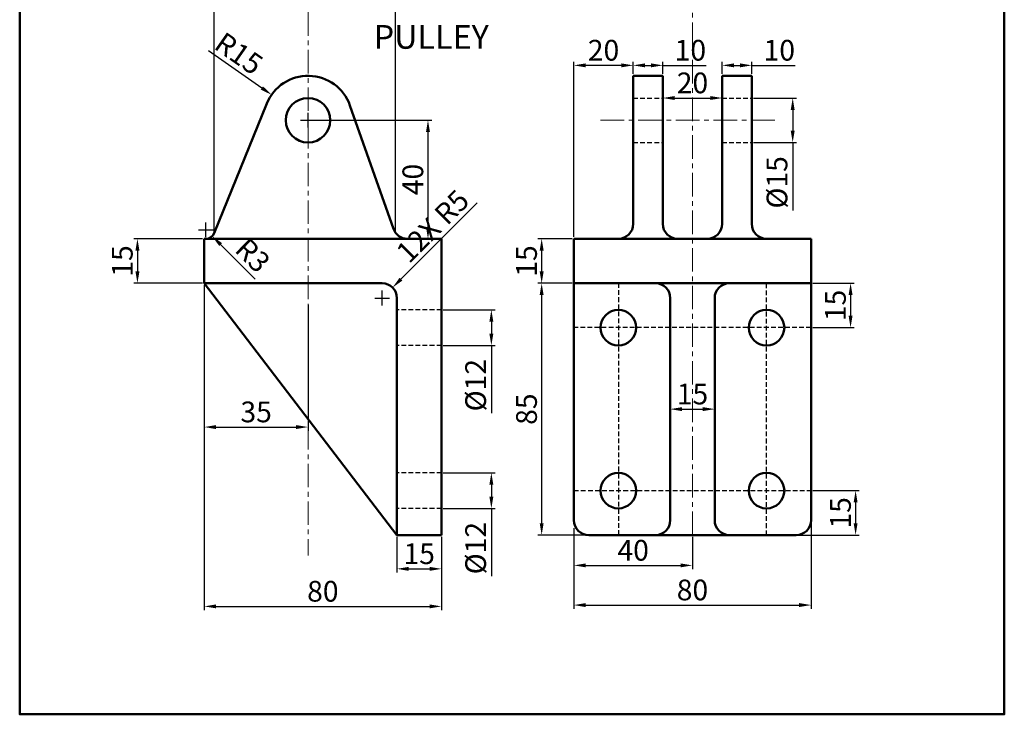
# Model space of a CAD drawing. Units: millimetres. Extents: x 50 to 393, y 3 to 474.
# Tile 1 of 2: x 61 to 393, y 3 to 238. Entities that reach past the tile are written whole.
import ezdxf

# ---------------------------------------------------------------- set-up
doc = ezdxf.new("R2010")
doc.units = ezdxf.units.MM
doc.header["$LTSCALE"] = 0.5
doc.linetypes.add('CENTER', pattern=[50.8, 31.75, -6.35, 6.35, -6.35])
doc.linetypes.add('HIDDEN', pattern=[9.525, 6.35, -3.175])
for name, color, linetype, lineweight in [('M-CNTR', 4, 'CENTER', 18), ('M-DIMS', 2, 'Continuous', 25), ('M-HIDN', 1, 'HIDDEN', 25), ('M-OUTL', 7, 'Continuous', 50), ('M-TEXT', 7, 'Continuous', 25), ('M-TTLB', 7, 'Continuous', 50)]:
    doc.layers.add(name, color=color, linetype=linetype, lineweight=lineweight)
doc.styles.get("Standard").update_dxf_attribs({"font": 'arial.ttf'})
doc.dimstyles.new('ISO-25', dxfattribs={"dimtxt": 7, "dimasz": 4, "dimexe": 1.25, "dimexo": 0.625, "dimtad": 1, "dimtxsty": 'Standard', "dimcen": 2.5, "dimadec": 0, "dimazin": 0, "dimtfac": 1, "dimtofl": 0, "dimtmove": 0, "dimatfit": 3, "dimfxl": 1, "dimarcsym": 0})

# ---------------------------------------------------------------- blocks, each defined once
blk = doc.blocks.new('*D1')
at = {"layer": 'Defpoints', "color": 0, "ltscale": 0.5, "transparency": 16777216}
for p in [(122.79, 163.96), (100.24, 148.96), (122.79, 148.96)]:
    blk.add_point(p, dxfattribs=at)
at = {"layer": 'M-DIMS', "color": 0, "lineweight": -2, "ltscale": 0.5, "transparency": 16777216}
for p, q in [((122.16, 163.96), (98.99, 163.96)), ((100.24, 159.96), (100.24, 152.96)), ((122.16, 148.96), (98.99, 148.96))]:
    blk.add_line(p, q, dxfattribs=at)
at = {"layer": 'M-DIMS', "color": 0, "ltscale": 0.5, "transparency": 16777216}
for points in [[(99.58, 159.96), (100.91, 159.96), (100.24, 163.96)], [(99.58, 152.96), (100.91, 152.96), (100.24, 148.96)]]:
    blk.add_solid(points, dxfattribs=at)
at = {"layer": 'M-DIMS', "color": 0, "ltscale": 0.5, "transparency": 16777216, "insert": (96.04, 156.46), "char_height": 7, "attachment_point": 5, "rotation": 90}
blk.add_mtext('15', dxfattribs=at)
blk = doc.blocks.new('*D2')
at = {"layer": 'Defpoints', "color": 0, "ltscale": 0.5, "transparency": 16777216}
for p in [(122.79, 148.96), (157.79, 142.23), (157.79, 100.41)]:
    blk.add_point(p, dxfattribs=at)
at = {"layer": 'M-DIMS', "color": 0, "lineweight": -2, "ltscale": 0.5, "transparency": 16777216}
for p, q in [((122.79, 148.34), (122.79, 99.16)), ((157.79, 141.61), (157.79, 99.16)), ((126.79, 100.41), (153.79, 100.41))]:
    blk.add_line(p, q, dxfattribs=at)
at = {"layer": 'M-DIMS', "color": 0, "ltscale": 0.5, "transparency": 16777216}
for points in [[(126.79, 101.07), (126.79, 99.74), (122.79, 100.41)], [(153.79, 101.07), (153.79, 99.74), (157.79, 100.41)]]:
    blk.add_solid(points, dxfattribs=at)
at = {"layer": 'M-DIMS', "color": 0, "ltscale": 0.5, "transparency": 16777216, "insert": (140.29, 104.61), "char_height": 7, "attachment_point": 5}
blk.add_mtext('35', dxfattribs=at)
blk = doc.blocks.new('*D3')
at = {"layer": 'Defpoints', "color": 0, "ltscale": 0.5, "transparency": 16777216}
for p in [(122.79, 148.96), (202.79, 63.96), (202.79, 39.89)]:
    blk.add_point(p, dxfattribs=at)
at = {"layer": 'M-DIMS', "color": 0, "lineweight": -2, "ltscale": 0.5, "transparency": 16777216}
for p, q in [((122.79, 148.34), (122.79, 38.64)), ((202.79, 63.34), (202.79, 38.64)), ((126.79, 39.89), (198.79, 39.89))]:
    blk.add_line(p, q, dxfattribs=at)
at = {"layer": 'M-DIMS', "color": 0, "ltscale": 0.5, "transparency": 16777216}
for points in [[(126.79, 40.55), (126.79, 39.22), (122.79, 39.89)], [(198.79, 40.55), (198.79, 39.22), (202.79, 39.89)]]:
    blk.add_solid(points, dxfattribs=at)
at = {"layer": 'M-DIMS', "color": 0, "ltscale": 0.5, "transparency": 16777216, "insert": (162.79, 44.09), "char_height": 7, "attachment_point": 5}
blk.add_mtext('80', dxfattribs=at)
blk = doc.blocks.new('*D4')
at = {"layer": 'Defpoints', "color": 0, "ltscale": 0.5, "transparency": 16777216}
for p in [(187.79, 63.96), (202.79, 63.96), (202.79, 52.56)]:
    blk.add_point(p, dxfattribs=at)
at = {"layer": 'M-DIMS', "color": 0, "lineweight": -2, "ltscale": 0.5, "transparency": 16777216}
for p, q in [((187.79, 63.34), (187.79, 51.31)), ((202.79, 63.34), (202.79, 51.31)), ((191.79, 52.56), (198.79, 52.56))]:
    blk.add_line(p, q, dxfattribs=at)
at = {"layer": 'M-DIMS', "color": 0, "ltscale": 0.5, "transparency": 16777216}
for points in [[(191.79, 53.23), (191.79, 51.89), (187.79, 52.56)], [(198.79, 53.23), (198.79, 51.89), (202.79, 52.56)]]:
    blk.add_solid(points, dxfattribs=at)
at = {"layer": 'M-DIMS', "color": 0, "ltscale": 0.5, "transparency": 16777216, "insert": (195.29, 56.76), "char_height": 7, "attachment_point": 5}
blk.add_mtext('15', dxfattribs=at)
blk = doc.blocks.new('*D5')
at = {"layer": 'Defpoints', "color": 0, "ltscale": 0.5, "transparency": 16777216}
for p in [(157.79, 203.96), (157.79, 163.96), (198.26, 163.96)]:
    blk.add_point(p, dxfattribs=at)
at = {"layer": 'M-DIMS', "color": 0, "lineweight": -2, "ltscale": 0.5, "transparency": 16777216}
for p, q in [((158.41, 203.96), (199.51, 203.96)), ((198.26, 199.96), (198.26, 167.96)), ((158.41, 163.96), (199.51, 163.96))]:
    blk.add_line(p, q, dxfattribs=at)
at = {"layer": 'M-DIMS', "color": 0, "ltscale": 0.5, "transparency": 16777216}
for points in [[(197.59, 199.96), (198.92, 199.96), (198.26, 203.96)], [(197.59, 167.96), (198.92, 167.96), (198.26, 163.96)]]:
    blk.add_solid(points, dxfattribs=at)
at = {"layer": 'M-DIMS', "color": 0, "ltscale": 0.5, "transparency": 16777216, "insert": (194.06, 183.96), "char_height": 7, "attachment_point": 5, "rotation": 90}
blk.add_mtext('40', dxfattribs=at)
blk = doc.blocks.new('*D6')
at = {"layer": 'Defpoints', "color": 0, "ltscale": 0.5, "transparency": 16777216}
for p in [(202.79, 139.96), (202.79, 127.96), (219.64, 127.96)]:
    blk.add_point(p, dxfattribs=at)
at = {"layer": 'M-DIMS', "color": 0, "lineweight": -2, "ltscale": 0.5, "transparency": 16777216}
for p, q in [((203.41, 139.96), (220.89, 139.96)), ((219.64, 135.96), (219.64, 131.96)), ((203.41, 127.96), (220.89, 127.96)), ((219.64, 127.96), (219.64, 105.14))]:
    blk.add_line(p, q, dxfattribs=at)
at = {"layer": 'M-DIMS', "color": 0, "ltscale": 0.5, "transparency": 16777216}
for points in [[(218.97, 135.96), (220.31, 135.96), (219.64, 139.96)], [(218.97, 131.96), (220.31, 131.96), (219.64, 127.96)]]:
    blk.add_solid(points, dxfattribs=at)
at = {"layer": 'M-DIMS', "color": 0, "ltscale": 0.5, "transparency": 16777216, "insert": (215.24, 114.55), "char_height": 7, "attachment_point": 5, "rotation": 90}
blk.add_mtext('%%C12', dxfattribs=at)
blk = doc.blocks.new('*D7')
at = {"layer": 'Defpoints', "color": 0, "ltscale": 0.5, "transparency": 16777216}
for p in [(202.79, 84.96), (202.79, 72.96), (219.64, 72.96)]:
    blk.add_point(p, dxfattribs=at)
at = {"layer": 'M-DIMS', "color": 0, "lineweight": -2, "ltscale": 0.5, "transparency": 16777216}
for p, q in [((203.41, 84.96), (220.89, 84.96)), ((219.64, 80.96), (219.64, 76.96)), ((203.41, 72.96), (220.89, 72.96)), ((219.64, 72.96), (219.64, 50.14))]:
    blk.add_line(p, q, dxfattribs=at)
at = {"layer": 'M-DIMS', "color": 0, "ltscale": 0.5, "transparency": 16777216}
for points in [[(218.97, 80.96), (220.31, 80.96), (219.64, 84.96)], [(218.97, 76.96), (220.31, 76.96), (219.64, 72.96)]]:
    blk.add_solid(points, dxfattribs=at)
at = {"layer": 'M-DIMS', "color": 0, "ltscale": 0.5, "transparency": 16777216, "insert": (215.24, 59.55), "char_height": 7, "attachment_point": 5, "rotation": 90}
blk.add_mtext('%%C12', dxfattribs=at)
blk = doc.blocks.new('*D8')
at = {"layer": 'Defpoints', "color": 0, "ltscale": 0.5, "transparency": 16777216}
for p in [(247.48, 163.96), (236.61, 148.96), (247.48, 148.96)]:
    blk.add_point(p, dxfattribs=at)
at = {"layer": 'M-DIMS', "color": 0, "lineweight": -2, "ltscale": 0.5, "transparency": 16777216}
for p, q in [((246.86, 163.96), (235.36, 163.96)), ((236.61, 159.96), (236.61, 152.96)), ((246.86, 148.96), (235.36, 148.96))]:
    blk.add_line(p, q, dxfattribs=at)
at = {"layer": 'M-DIMS', "color": 0, "ltscale": 0.5, "transparency": 16777216}
for points in [[(235.94, 159.96), (237.28, 159.96), (236.61, 163.96)], [(235.94, 152.96), (237.28, 152.96), (236.61, 148.96)]]:
    blk.add_solid(points, dxfattribs=at)
at = {"layer": 'M-DIMS', "color": 0, "ltscale": 0.5, "transparency": 16777216, "insert": (232.41, 156.46), "char_height": 7, "attachment_point": 5, "rotation": 90}
blk.add_mtext('15', dxfattribs=at)
blk = doc.blocks.new('*D9')
at = {"layer": 'Defpoints', "color": 0, "ltscale": 0.5, "transparency": 16777216}
for p in [(247.48, 148.96), (236.61, 63.96), (252.48, 63.96)]:
    blk.add_point(p, dxfattribs=at)
at = {"layer": 'M-DIMS', "color": 0, "lineweight": -2, "ltscale": 0.5, "transparency": 16777216}
for p, q in [((246.86, 148.96), (235.36, 148.96)), ((236.61, 144.96), (236.61, 67.96)), ((251.86, 63.96), (235.36, 63.96))]:
    blk.add_line(p, q, dxfattribs=at)
at = {"layer": 'M-DIMS', "color": 0, "ltscale": 0.5, "transparency": 16777216}
for points in [[(235.94, 144.96), (237.28, 144.96), (236.61, 148.96)], [(235.94, 67.96), (237.28, 67.96), (236.61, 63.96)]]:
    blk.add_solid(points, dxfattribs=at)
at = {"layer": 'M-DIMS', "color": 0, "ltscale": 0.5, "transparency": 16777216, "insert": (232.41, 106.46), "char_height": 7, "attachment_point": 5, "rotation": 90}
blk.add_mtext('85', dxfattribs=at)
blk = doc.blocks.new('*D10')
at = {"layer": 'Defpoints', "color": 0, "ltscale": 0.5, "transparency": 16777216}
for p in [(247.48, 63.96), (287.48, 63.96), (287.48, 53.73)]:
    blk.add_point(p, dxfattribs=at)
at = {"layer": 'M-DIMS', "color": 0, "lineweight": -2, "ltscale": 0.5, "transparency": 16777216}
for p, q in [((247.48, 63.34), (247.48, 52.48)), ((287.48, 63.34), (287.48, 52.48)), ((251.48, 53.73), (283.48, 53.73))]:
    blk.add_line(p, q, dxfattribs=at)
at = {"layer": 'M-DIMS', "color": 0, "ltscale": 0.5, "transparency": 16777216}
for points in [[(251.48, 54.39), (251.48, 53.06), (247.48, 53.73)], [(283.48, 54.39), (283.48, 53.06), (287.48, 53.73)]]:
    blk.add_solid(points, dxfattribs=at)
at = {"layer": 'M-DIMS', "color": 0, "ltscale": 0.5, "transparency": 16777216, "insert": (267.48, 57.92), "char_height": 7, "attachment_point": 5}
blk.add_mtext('40', dxfattribs=at)
blk = doc.blocks.new('*D11')
at = {"layer": 'Defpoints', "color": 0, "ltscale": 0.5, "transparency": 16777216}
for p in [(247.48, 66.89), (327.48, 68.96), (327.48, 40.33)]:
    blk.add_point(p, dxfattribs=at)
at = {"layer": 'M-DIMS', "color": 0, "lineweight": -2, "ltscale": 0.5, "transparency": 16777216}
for p, q in [((327.48, 68.34), (327.48, 39.08)), ((247.48, 66.27), (247.48, 39.08)), ((251.48, 40.33), (323.48, 40.33))]:
    blk.add_line(p, q, dxfattribs=at)
at = {"layer": 'M-DIMS', "color": 0, "ltscale": 0.5, "transparency": 16777216}
for points in [[(251.48, 41), (251.48, 39.67), (247.48, 40.33)], [(323.48, 41), (323.48, 39.67), (327.48, 40.33)]]:
    blk.add_solid(points, dxfattribs=at)
at = {"layer": 'M-DIMS', "color": 0, "ltscale": 0.5, "transparency": 16777216, "insert": (287.48, 44.53), "char_height": 7, "attachment_point": 5}
blk.add_mtext('80', dxfattribs=at)
blk = doc.blocks.new('*D12')
at = {"layer": 'Defpoints', "color": 0, "ltscale": 0.5, "transparency": 16777216}
for p in [(327.48, 148.96), (327.48, 133.96), (340.82, 133.96)]:
    blk.add_point(p, dxfattribs=at)
at = {"layer": 'M-DIMS', "color": 0, "lineweight": -2, "ltscale": 0.5, "transparency": 16777216}
for p, q in [((328.11, 148.96), (342.07, 148.96)), ((340.82, 144.96), (340.82, 137.96)), ((328.11, 133.96), (342.07, 133.96))]:
    blk.add_line(p, q, dxfattribs=at)
at = {"layer": 'M-DIMS', "color": 0, "ltscale": 0.5, "transparency": 16777216}
for points in [[(340.16, 144.96), (341.49, 144.96), (340.82, 148.96)], [(340.16, 137.96), (341.49, 137.96), (340.82, 133.96)]]:
    blk.add_solid(points, dxfattribs=at)
at = {"layer": 'M-DIMS', "color": 0, "ltscale": 0.5, "transparency": 16777216, "insert": (336.62, 141.46), "char_height": 7, "attachment_point": 5, "rotation": 90}
blk.add_mtext('15', dxfattribs=at)
blk = doc.blocks.new('*D13')
at = {"layer": 'Defpoints', "color": 0, "ltscale": 0.5, "transparency": 16777216}
for p in [(279.98, 106.46), (294.98, 106.46), (294.98, 106.46)]:
    blk.add_point(p, dxfattribs=at)
at = {"layer": 'M-DIMS', "color": 0, "lineweight": -2, "ltscale": 0.5, "transparency": 16777216}
for p, q in [((279.98, 107.09), (279.98, 107.71)), ((283.98, 106.46), (290.98, 106.46)), ((294.98, 107.09), (294.98, 107.71))]:
    blk.add_line(p, q, dxfattribs=at)
at = {"layer": 'M-DIMS', "color": 0, "ltscale": 0.5, "transparency": 16777216}
for points in [[(283.98, 107.13), (283.98, 105.8), (279.98, 106.46)], [(290.98, 107.13), (290.98, 105.8), (294.98, 106.46)]]:
    blk.add_solid(points, dxfattribs=at)
at = {"layer": 'M-DIMS', "color": 0, "ltscale": 0.5, "transparency": 16777216, "insert": (287.48, 110.66), "char_height": 7, "attachment_point": 5}
blk.add_mtext('15', dxfattribs=at)
blk = doc.blocks.new('*D14')
at = {"layer": 'Defpoints', "color": 0, "ltscale": 0.5, "transparency": 16777216}
for p in [(327.48, 78.96), (312.48, 63.96), (342.52, 63.96)]:
    blk.add_point(p, dxfattribs=at)
at = {"layer": 'M-DIMS', "color": 0, "lineweight": -2, "ltscale": 0.5, "transparency": 16777216}
for p, q in [((328.11, 78.96), (343.77, 78.96)), ((342.52, 74.96), (342.52, 67.96)), ((313.11, 63.96), (343.77, 63.96))]:
    blk.add_line(p, q, dxfattribs=at)
at = {"layer": 'M-DIMS', "color": 0, "ltscale": 0.5, "transparency": 16777216}
for points in [[(341.85, 74.96), (343.18, 74.96), (342.52, 78.96)], [(341.85, 67.96), (343.18, 67.96), (342.52, 63.96)]]:
    blk.add_solid(points, dxfattribs=at)
at = {"layer": 'M-DIMS', "color": 0, "ltscale": 0.5, "transparency": 16777216, "insert": (338.32, 71.46), "char_height": 7, "attachment_point": 5, "rotation": 90}
blk.add_mtext('15', dxfattribs=at)
blk = doc.blocks.new('*D15')
at = {"layer": 'Defpoints', "color": 0, "ltscale": 0.5, "transparency": 16777216}
for p in [(307.48, 211.46), (307.48, 196.46), (321.3, 196.46)]:
    blk.add_point(p, dxfattribs=at)
at = {"layer": 'M-DIMS', "color": 0, "lineweight": -2, "ltscale": 0.5, "transparency": 16777216}
for p, q in [((308.11, 211.46), (322.55, 211.46)), ((321.3, 207.46), (321.3, 200.46)), ((308.11, 196.46), (322.55, 196.46)), ((321.3, 196.46), (321.3, 173.52))]:
    blk.add_line(p, q, dxfattribs=at)
at = {"layer": 'M-DIMS', "color": 0, "ltscale": 0.5, "transparency": 16777216}
for points in [[(320.63, 207.46), (321.96, 207.46), (321.3, 211.46)], [(320.63, 200.46), (321.96, 200.46), (321.3, 196.46)]]:
    blk.add_solid(points, dxfattribs=at)
at = {"layer": 'M-DIMS', "color": 0, "ltscale": 0.5, "transparency": 16777216, "insert": (316.9, 182.99), "char_height": 7, "attachment_point": 5, "rotation": 90}
blk.add_mtext('%%C15', dxfattribs=at)
blk = doc.blocks.new('*D16')
at = {"layer": 'Defpoints', "color": 0, "ltscale": 0.5, "transparency": 16777216}
for p in [(247.48, 222.48), (267.48, 218.96), (247.48, 163.96)]:
    blk.add_point(p, dxfattribs=at)
at = {"layer": 'M-DIMS', "color": 0, "lineweight": -2, "ltscale": 0.5, "transparency": 16777216}
for p, q in [((247.48, 164.59), (247.48, 223.73)), ((267.48, 219.59), (267.48, 223.73)), ((263.48, 222.48), (251.48, 222.48))]:
    blk.add_line(p, q, dxfattribs=at)
at = {"layer": 'M-DIMS', "color": 0, "ltscale": 0.5, "transparency": 16777216}
for points in [[(251.48, 223.15), (251.48, 221.82), (247.48, 222.48)], [(263.48, 223.15), (263.48, 221.82), (267.48, 222.48)]]:
    blk.add_solid(points, dxfattribs=at)
at = {"layer": 'M-DIMS', "color": 0, "ltscale": 0.5, "transparency": 16777216, "insert": (257.48, 226.68), "char_height": 7, "attachment_point": 5}
blk.add_mtext('20', dxfattribs=at)
blk = doc.blocks.new('*D17')
at = {"layer": 'Defpoints', "color": 0, "ltscale": 0.5, "transparency": 16777216}
for p in [(277.48, 222.48), (267.48, 218.96), (277.48, 218.96)]:
    blk.add_point(p, dxfattribs=at)
at = {"layer": 'M-DIMS', "color": 0, "lineweight": -2, "ltscale": 0.5, "transparency": 16777216}
for p, q in [((267.48, 219.59), (267.48, 223.73)), ((277.48, 219.59), (277.48, 223.73)), ((271.48, 222.48), (273.48, 222.48)), ((277.48, 222.48), (292.08, 222.48))]:
    blk.add_line(p, q, dxfattribs=at)
at = {"layer": 'M-DIMS', "color": 0, "ltscale": 0.5, "transparency": 16777216}
for points in [[(271.48, 223.15), (271.48, 221.82), (267.48, 222.48)], [(273.48, 223.15), (273.48, 221.82), (277.48, 222.48)]]:
    blk.add_solid(points, dxfattribs=at)
at = {"layer": 'M-DIMS', "color": 0, "ltscale": 0.5, "transparency": 16777216, "insert": (286.78, 226.68), "char_height": 7, "attachment_point": 5}
blk.add_mtext('10', dxfattribs=at)
blk = doc.blocks.new('*D18')
at = {"layer": 'Defpoints', "color": 0, "ltscale": 0.5, "transparency": 16777216}
for p in [(277.48, 218.96), (297.48, 218.96), (297.48, 211.46)]:
    blk.add_point(p, dxfattribs=at)
at = {"layer": 'M-DIMS', "color": 0, "lineweight": -2, "ltscale": 0.5, "transparency": 16777216}
for p, q in [((277.48, 218.34), (277.48, 210.21)), ((297.48, 218.34), (297.48, 210.21)), ((281.48, 211.46), (293.48, 211.46))]:
    blk.add_line(p, q, dxfattribs=at)
at = {"layer": 'M-DIMS', "color": 0, "ltscale": 0.5, "transparency": 16777216}
for points in [[(281.48, 212.13), (281.48, 210.8), (277.48, 211.46)], [(293.48, 212.13), (293.48, 210.8), (297.48, 211.46)]]:
    blk.add_solid(points, dxfattribs=at)
at = {"layer": 'M-DIMS', "color": 0, "ltscale": 0.5, "transparency": 16777216, "insert": (287.48, 215.66), "char_height": 7, "attachment_point": 5}
blk.add_mtext('20', dxfattribs=at)
blk = doc.blocks.new('*D19')
at = {"layer": 'Defpoints', "color": 0, "ltscale": 0.5, "transparency": 16777216}
for p in [(307.48, 222.48), (297.48, 218.96), (307.48, 218.96)]:
    blk.add_point(p, dxfattribs=at)
at = {"layer": 'M-DIMS', "color": 0, "lineweight": -2, "ltscale": 0.5, "transparency": 16777216}
for p, q in [((297.48, 219.59), (297.48, 223.73)), ((307.48, 219.59), (307.48, 223.73)), ((301.48, 222.48), (303.48, 222.48)), ((307.48, 222.48), (322.08, 222.48))]:
    blk.add_line(p, q, dxfattribs=at)
at = {"layer": 'M-DIMS', "color": 0, "ltscale": 0.5, "transparency": 16777216}
for points in [[(301.48, 223.15), (301.48, 221.82), (297.48, 222.48)], [(303.48, 223.15), (303.48, 221.82), (307.48, 222.48)]]:
    blk.add_solid(points, dxfattribs=at)
at = {"layer": 'M-DIMS', "color": 0, "ltscale": 0.5, "transparency": 16777216, "insert": (316.78, 226.68), "char_height": 7, "attachment_point": 5}
blk.add_mtext('10', dxfattribs=at)
blk = doc.blocks.new('*D36')
at = {"layer": 'Defpoints', "color": 0, "ltscale": 0.5, "transparency": 16777216}
for p in [(145.49, 212.56), (157.79, 203.96)]:
    blk.add_point(p, dxfattribs=at)
at = {"layer": 'M-DIMS', "color": 0, "lineweight": -2, "ltscale": 0.5, "transparency": 16777216}
for p, q in [((124.16, 227.47), (142.22, 214.85)), ((157.79, 201.46), (157.79, 206.46)), ((155.29, 203.96), (160.29, 203.96))]:
    blk.add_line(p, q, dxfattribs=at)
at = {"layer": 'M-DIMS', "color": 0, "ltscale": 0.5, "transparency": 16777216}
blk.add_solid([(142.6, 215.4), (141.83, 214.3), (145.49, 212.56)], dxfattribs=at)
at = {"layer": 'M-DIMS', "color": 0, "ltscale": 0.5, "transparency": 16777216, "insert": (133.96, 225.75), "char_height": 7, "attachment_point": 5, "rotation": 325.0399}
blk.add_mtext('R15', dxfattribs=at)
blk = doc.blocks.new('*D40')
at = {"layer": 'Defpoints', "color": 0, "ltscale": 0.5, "transparency": 16777216}
for p in [(187.35, 422.96), (126.11, 165.84), (187.35, 165.94)]:
    blk.add_point(p, dxfattribs=at)
at = {"layer": 'M-DIMS', "color": 0, "lineweight": -2, "ltscale": 0.5, "transparency": 16777216}
for p, q in [((126.11, 166.46), (126.11, 424.21)), ((130.11, 422.96), (183.35, 422.96)), ((187.35, 166.56), (187.35, 424.21))]:
    blk.add_line(p, q, dxfattribs=at)
at = {"layer": 'M-DIMS', "color": 0, "ltscale": 0.5, "transparency": 16777216}
for points in [[(130.11, 423.63), (130.11, 422.29), (126.11, 422.96)], [(183.35, 423.63), (183.35, 422.29), (187.35, 422.96)]]:
    blk.add_solid(points, dxfattribs=at)
at = {"layer": 'M-DIMS', "color": 0, "ltscale": 0.5, "transparency": 16777216, "insert": (156.73, 427.16), "char_height": 7, "attachment_point": 5}
blk.add_mtext('61.24', dxfattribs=at)
blk = doc.blocks.new('*D41')
at = {"layer": 'Defpoints', "color": 0, "ltscale": 0.5, "transparency": 16777216}
for p in [(186.32, 147.5), (182.79, 143.96)]:
    blk.add_point(p, dxfattribs=at)
at = {"layer": 'M-DIMS', "color": 0, "lineweight": -2, "ltscale": 0.5, "transparency": 16777216}
for p, q in [((214.89, 176.08), (189.15, 150.33)), ((182.79, 141.46), (182.79, 146.46)), ((180.29, 143.96), (185.29, 143.96))]:
    blk.add_line(p, q, dxfattribs=at)
at = {"layer": 'M-DIMS', "color": 0, "ltscale": 0.5, "transparency": 16777216}
blk.add_solid([(188.68, 150.8), (189.62, 149.86), (186.32, 147.5)], dxfattribs=at)
at = {"layer": 'M-DIMS', "color": 0, "ltscale": 0.5, "transparency": 16777216, "insert": (200.47, 167.59), "char_height": 7, "attachment_point": 5, "rotation": 45.0042}
blk.add_mtext('12X R5', dxfattribs=at)
blk = doc.blocks.new('*D42')
at = {"layer": 'Defpoints', "color": 0, "ltscale": 0.5, "transparency": 16777216}
for p in [(123.33, 166.96), (125.45, 164.85)]:
    blk.add_point(p, dxfattribs=at)
at = {"layer": 'M-DIMS', "color": 0, "lineweight": -2, "ltscale": 0.5, "transparency": 16777216}
for p, q in [((123.33, 164.46), (123.33, 169.46)), ((120.83, 166.96), (125.83, 166.96)), ((140, 150.35), (128.29, 162.02))]:
    blk.add_line(p, q, dxfattribs=at)
at = {"layer": 'M-DIMS', "color": 0, "ltscale": 0.5, "transparency": 16777216}
blk.add_solid([(128.76, 162.5), (127.82, 161.55), (125.45, 164.85)], dxfattribs=at)
at = {"layer": 'M-DIMS', "color": 0, "ltscale": 0.5, "transparency": 16777216, "insert": (138.53, 157.75), "char_height": 7, "attachment_point": 5, "rotation": 315.1036}
blk.add_mtext('R3', dxfattribs=at)

msp = doc.modelspace()

# ---------------------------------------------------------------- linework, layer by layer
at = {"layer": 'M-CNTR', "ltscale": 0.5}
for p, q in [((287.481, 63.964), (287.481, 337.045)), ((157.787, 303.93), (157.787, 57.07)), ((256.495, 203.964), (316.384, 203.964))]:
    msp.add_line(p, q, dxfattribs=at)
at = {"layer": 'M-HIDN', "ltscale": 0.5}
for p, q in [((267.481, 211.464), (277.481, 211.464)), ((297.481, 211.464), (307.481, 211.464)), ((267.481, 196.464), (277.481, 196.464)), ((297.481, 196.464), (307.481, 196.464)), ((262.481, 148.964), (262.481, 63.964)), ((312.481, 63.964), (312.481, 148.964)), ((202.787, 139.964), (187.787, 139.964)), ((327.481, 133.964), (247.481, 133.964)), ((202.787, 127.964), (187.787, 127.964)), ((202.787, 84.964), (187.787, 84.964)), ((247.481, 78.964), (327.481, 78.964)), ((202.787, 72.964), (187.787, 72.964))]:
    msp.add_line(p, q, dxfattribs=at)
at = {"layer": 'M-OUTL', "ltscale": 0.5}
for p, q in [((267.481, 218.964), (277.481, 218.964)), ((267.481, 168.964), (267.481, 218.964)), ((277.481, 168.964), (277.481, 218.964)), ((297.481, 168.964), (297.481, 218.964)), ((297.481, 218.964), (307.481, 218.964)), ((307.481, 168.964), (307.481, 218.964)), ((143.889, 209.609), (126.108, 165.835)), ((171.934, 208.95), (186.61, 167.302)), ((247.481, 163.964), (247.481, 68.964)), ((262.481, 163.964), (247.481, 163.964)), ((312.481, 163.964), (262.481, 163.964)), ((327.481, 163.964), (287.481, 163.964)), ((327.481, 68.964), (327.481, 163.964)), ((274.981, 148.964), (247.481, 148.964)), ((327.481, 148.964), (274.981, 148.964)), ((279.981, 68.964), (279.981, 143.964)), ((294.981, 68.964), (294.981, 143.964)), ((252.481, 63.964), (299.981, 63.964)), ((299.981, 63.964), (322.481, 63.964))]:
    msp.add_line(p, q, dxfattribs=at)
at = {"layer": 'M-OUTL'}
for p, q in [((123.008, 163.964), (122.787, 163.964)), ((122.787, 163.964), (122.787, 148.964)), ((123.329, 163.964), (123.008, 163.964)), ((191.326, 163.964), (123.329, 163.964)), ((202.787, 163.964), (191.326, 163.964)), ((202.787, 63.964), (202.787, 163.964)), ((122.787, 148.964), (182.787, 148.964)), ((187.787, 63.964), (122.787, 148.964)), ((187.787, 143.964), (187.787, 63.964)), ((187.787, 63.964), (202.787, 63.964))]:
    msp.add_line(p, q, dxfattribs=at)
at = {"layer": 'M-OUTL', "ltscale": 0.5}
for centre, radius in [((157.787, 203.964), 7.5), ((262.481, 133.964), 6), ((312.481, 133.964), 6), ((262.481, 78.964), 6), ((312.481, 78.964), 6)]:
    msp.add_circle(centre, radius, dxfattribs=at)
for centre, radius, start, end in [((157.787, 203.964), 15, 19.41229, 157.89295), ((262.481, 168.964), 5, 270, 0), ((282.481, 168.964), 5, 180, 270), ((292.481, 168.964), 5, 270, 0), ((312.481, 168.964), 5, 180, 270), ((123.329, 166.964), 3, 270, 337.89295), ((274.981, 143.964), 5, 0, 90), ((299.981, 143.964), 5, 90, 180), ((252.481, 68.964), 5, 180, 270), ((274.981, 68.964), 5, 270, 0), ((299.981, 68.964), 5, 180, 270), ((322.481, 68.964), 5, 270, 0)]:
    msp.add_arc(centre, radius, start, end, dxfattribs=at)
at = {"layer": 'M-OUTL'}
for centre, start, end in [((191.326, 168.964), 199.41229, 270), ((182.787, 143.964), 360, 90)]:
    msp.add_arc(centre, 5, start, end, dxfattribs=at)
at = {"layer": 'M-TTLB', "ltscale": 0.5}
msp.add_lwpolyline([(60.52, 474.222), (392.686, 474.222), (392.686, 3.466), (60.52, 3.466)], close=True, dxfattribs=at)

# ---------------------------------------------------------------- texts
at = {"layer": 'M-TEXT', "ltscale": 0.5, "insert": (179.936, 236.091), "char_height": 8, "attachment_point": 1}
msp.add_mtext_dynamic_manual_height_columns('PULLEY', width=45.18848, gutter_width=12.5, heights=[0], dxfattribs=at)

# ---------------------------------------------------------------- dimensions: what is measured, and where the dimension line sits
at = {"layer": 'M-DIMS', "ltscale": 0.5}
for base, p1, p2, override, picture, middle in [((187.346, 422.958), (126.108, 165.835), (187.346, 165.937), {"dimdec": 2, "dimlfac": 1, "dimrnd": 0, "dimzin": 0, "dimdsep": 46, "dimlunit": 2}, '*D40', (156.727, 427.157)), ((247.481, 222.483), (267.481, 218.964), (247.481, 163.964), {"dimclrd": 0, "dimclre": 0, "dimclrt": 0}, '*D16', (257.481, 226.682)), ((277.481, 222.483), (267.481, 218.964), (277.481, 218.964), {"dimclrd": 0, "dimclre": 0, "dimclrt": 0}, '*D17', (286.779, 226.682)), ((307.481, 222.483), (297.481, 218.964), (307.481, 218.964), {"dimclrd": 0, "dimclre": 0, "dimclrt": 0}, '*D19', (316.779, 226.682)), ((297.481, 211.464), (277.481, 218.964), (297.481, 218.964), {"dimclrd": 0, "dimclre": 0, "dimclrt": 0}, '*D18', (287.481, 215.663)), ((157.787, 100.407), (122.787, 148.964), (157.787, 142.232), {"dimclrd": 0, "dimclre": 0, "dimclrt": 0}, '*D2', (140.287, 104.609)), ((202.787, 39.887), (122.787, 148.964), (202.787, 63.964), {"dimclrd": 0, "dimclre": 0, "dimclrt": 0}, '*D3', (162.787, 44.086)), ((294.981, 106.464), (279.981, 106.464), (294.981, 106.464), {"dimclrd": 0, "dimclre": 0, "dimclrt": 0}, '*D13', (287.481, 110.663)), ((327.481, 40.332), (247.481, 66.893), (327.481, 68.964), {"dimclrd": 0, "dimclre": 0, "dimclrt": 0}, '*D11', (287.481, 44.531)), ((287.481, 53.726), (247.481, 63.964), (287.481, 63.964), {"dimclrd": 0, "dimclre": 0, "dimclrt": 0}, '*D10', (267.481, 57.925))]:
    dim = msp.add_linear_dim(base=base, p1=p1, p2=p2, dimstyle='ISO-25', override=override, dxfattribs=at)
    dim.commit()
    dim.dimension.update_dxf_attribs({"geometry": picture, "text_midpoint": middle})
for center, mpoint, override, picture, middle in [((157.787, 203.964), (145.493, 212.559), {"dimclrd": 0, "dimclre": 0, "dimclrt": 0}, '*D36', (133.955, 225.75)), ((123.329, 166.964), (125.454, 164.847), {"dimdec": 0, "dimlfac": 1, "dimrnd": 0, "dimzin": 0, "dimdsep": 46, "dimlunit": 2}, '*D42', (138.527, 157.751))]:
    dim = msp.add_radius_dim(center=center, mpoint=mpoint, dimstyle='ISO-25', override=override, dxfattribs=at)
    dim.commit()
    dim.dimension.update_dxf_attribs({"geometry": picture, "text_midpoint": middle})
for base, p1, p2, picture, middle in [((321.298, 196.464), (307.481, 211.464), (307.481, 196.464), '*D15', (316.903, 182.991)), ((219.639, 127.964), (202.787, 139.964), (202.787, 127.964), '*D6', (215.244, 114.553)), ((219.639, 72.964), (202.787, 84.964), (202.787, 72.964), '*D7', (215.244, 59.553))]:
    dim = msp.add_linear_dim(base=base, p1=p1, p2=p2, angle=90, text='%%C<>', dimstyle='ISO-25', override={"dimclrd": 0, "dimclre": 0, "dimclrt": 0}, dxfattribs=at)
    dim.commit()
    dim.dimension.update_dxf_attribs({"geometry": picture, "text_midpoint": middle})
for base, p1, p2, picture, middle in [((198.256, 163.964), (157.787, 203.964), (157.787, 163.964), '*D5', (194.057, 183.964)), ((100.244, 148.964), (122.787, 163.964), (122.787, 148.964), '*D1', (96.045, 156.464)), ((236.609, 148.964), (247.481, 163.964), (247.481, 148.964), '*D8', (232.41, 156.464)), ((236.609, 63.964), (247.481, 148.964), (252.481, 63.964), '*D9', (232.41, 106.464)), ((340.824, 133.964), (327.481, 148.964), (327.481, 133.964), '*D12', (336.625, 141.464)), ((342.516, 63.964), (327.481, 78.964), (312.481, 63.964), '*D14', (338.317, 71.464))]:
    dim = msp.add_linear_dim(base=base, p1=p1, p2=p2, angle=90, dimstyle='ISO-25', override={"dimclrd": 0, "dimclre": 0, "dimclrt": 0}, dxfattribs=at)
    dim.commit()
    dim.dimension.update_dxf_attribs({"geometry": picture, "text_midpoint": middle})
dim = msp.add_radius_dim(center=(182.787, 143.964), mpoint=(186.322, 147.5), text='12X <>', dimstyle='ISO-25', override={"dimdec": 0, "dimlfac": 1, "dimrnd": 0, "dimzin": 0, "dimdsep": 46, "dimlunit": 2}, dxfattribs=at)
dim.commit()
dim.dimension.update_dxf_attribs({"geometry": '*D41', "text_midpoint": (200.467, 167.586)})
dim = msp.add_linear_dim(base=(202.787, 52.559), p1=(187.787, 63.964), p2=(202.787, 63.964), dimstyle='ISO-25', override={"dimclrd": 0, "dimclre": 0, "dimclrt": 0}, dxfattribs=at)
dim.commit()
dim.dimension.update_dxf_attribs({"geometry": '*D4', "text_midpoint": (195.287, 52.559), "dimtype": 160})

doc.saveas('drawing.dxf')
